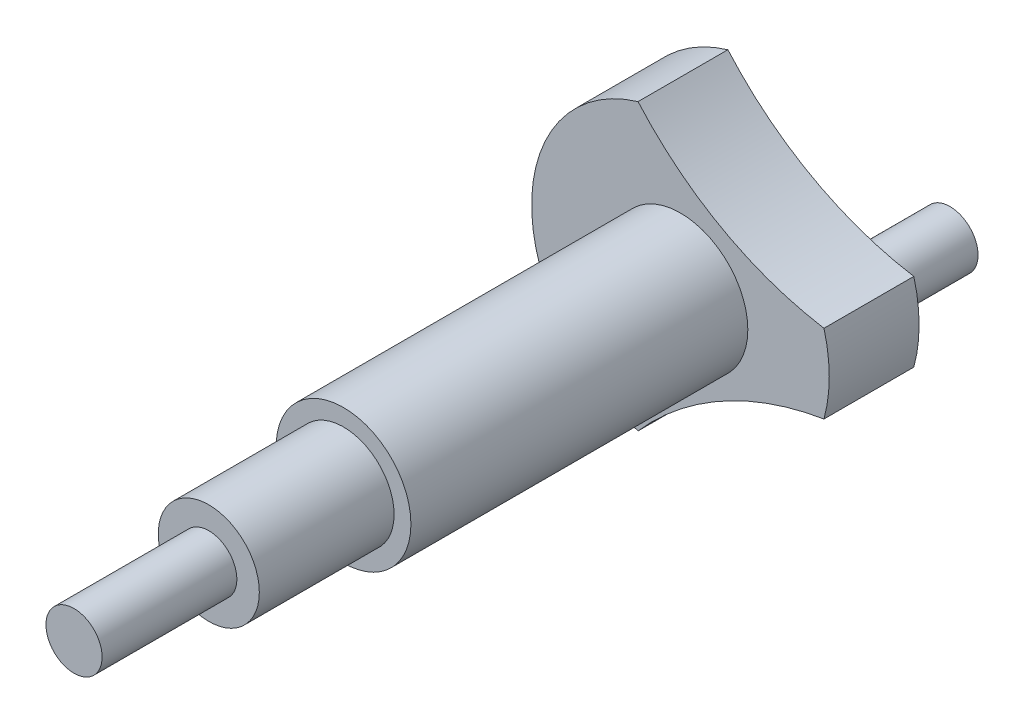
ISO-10303-21;
HEADER;
FILE_DESCRIPTION(('STEP AP214'),'2;1');
FILE_NAME('part.step','',(''),(''),'','','');
FILE_SCHEMA(('AUTOMOTIVE_DESIGN { 1 0 10303 214 1 1 1 1 }'));
ENDSEC;
DATA;
#1=APPLICATION_CONTEXT('core data for automotive mechanical design processes');
#2=APPLICATION_PROTOCOL_DEFINITION('international standard','automotive_design',2000,#1);
#3=PRODUCT_CONTEXT('',#1,'mechanical');
#4=PRODUCT('Part','Part','',(#3));
#5=PRODUCT_RELATED_PRODUCT_CATEGORY('part','',(#4));
#6=PRODUCT_DEFINITION_FORMATION('','',#4);
#7=PRODUCT_DEFINITION_CONTEXT('part definition',#1,'design');
#8=PRODUCT_DEFINITION('design','',#6,#7);
#9=PRODUCT_DEFINITION_SHAPE('','',#8);
#10=(LENGTH_UNIT() NAMED_UNIT(*) SI_UNIT(.MILLI.,.METRE.));
#11=(NAMED_UNIT(*) PLANE_ANGLE_UNIT() SI_UNIT($,.RADIAN.));
#12=(NAMED_UNIT(*) SI_UNIT($,.STERADIAN.) SOLID_ANGLE_UNIT());
#13=UNCERTAINTY_MEASURE_WITH_UNIT(LENGTH_MEASURE(1.E-05),#10,'distance_accuracy_value','');
#14=(GEOMETRIC_REPRESENTATION_CONTEXT(3) GLOBAL_UNCERTAINTY_ASSIGNED_CONTEXT((#13)) GLOBAL_UNIT_ASSIGNED_CONTEXT((#10,
#11,#12)) REPRESENTATION_CONTEXT('',''));
#15=CARTESIAN_POINT('',(0.,0.,0.));
#16=DIRECTION('',(0.,0.,1.));
#17=DIRECTION('',(1.,0.,0.));
#18=AXIS2_PLACEMENT_3D('',#15,#16,#17);
#19=CARTESIAN_POINT('',(0.,0.,30.));
#20=DIRECTION('',(0.,0.,-1.));
#21=DIRECTION('',(-1.,0.,0.));
#22=AXIS2_PLACEMENT_3D('',#19,#20,#21);
#23=CYLINDRICAL_SURFACE('',#22,6.);
#24=CARTESIAN_POINT('',(0.,0.,30.));
#25=DIRECTION('',(0.,0.,1.));
#26=DIRECTION('',(1.,0.,0.));
#27=AXIS2_PLACEMENT_3D('',#24,#25,#26);
#28=CIRCLE('',#27,6.);
#29=CARTESIAN_POINT('',(6.,0.,30.));
#30=VERTEX_POINT('',#29);
#31=EDGE_CURVE('E123',#30,#30,#28,.T.);
#32=ORIENTED_EDGE('',*,*,#31,.F.);
#33=EDGE_LOOP('',(#32));
#34=FACE_BOUND('',#33,.T.);
#35=CARTESIAN_POINT('',(0.,0.,0.));
#36=DIRECTION('',(0.,0.,1.));
#37=DIRECTION('',(1.,0.,0.));
#38=AXIS2_PLACEMENT_3D('',#35,#36,#37);
#39=CIRCLE('',#38,6.);
#40=CARTESIAN_POINT('',(6.,0.,0.));
#41=VERTEX_POINT('',#40);
#42=EDGE_CURVE('E45',#41,#41,#39,.T.);
#43=ORIENTED_EDGE('',*,*,#42,.T.);
#44=EDGE_LOOP('',(#43));
#45=FACE_BOUND('',#44,.T.);
#46=ADVANCED_FACE('F39',(#34,#45),#23,.T.);
#47=CARTESIAN_POINT('',(0.,0.,30.));
#48=DIRECTION('',(0.,0.,1.));
#49=DIRECTION('',(1.,0.,0.));
#50=AXIS2_PLACEMENT_3D('',#47,#48,#49);
#51=PLANE('',#50);
#52=CARTESIAN_POINT('',(0.,0.,30.));
#53=DIRECTION('',(0.,0.,1.));
#54=DIRECTION('',(1.,0.,0.));
#55=AXIS2_PLACEMENT_3D('',#52,#53,#54);
#56=CIRCLE('',#55,4.5);
#57=CARTESIAN_POINT('',(4.5,0.,30.));
#58=VERTEX_POINT('',#57);
#59=EDGE_CURVE('E48',#58,#58,#56,.T.);
#60=ORIENTED_EDGE('',*,*,#59,.F.);
#61=EDGE_LOOP('',(#60));
#62=FACE_BOUND('',#61,.T.);
#63=ORIENTED_EDGE('',*,*,#31,.T.);
#64=EDGE_LOOP('',(#63));
#65=FACE_BOUND('',#64,.T.);
#66=ADVANCED_FACE('F129',(#62,#65),#51,.T.);
#67=CARTESIAN_POINT('',(0.,0.,42.));
#68=DIRECTION('',(0.,0.,-1.));
#69=DIRECTION('',(-1.,0.,0.));
#70=AXIS2_PLACEMENT_3D('',#67,#68,#69);
#71=CYLINDRICAL_SURFACE('',#70,4.5);
#72=CARTESIAN_POINT('',(0.,0.,42.));
#73=DIRECTION('',(0.,0.,1.));
#74=DIRECTION('',(1.,0.,0.));
#75=AXIS2_PLACEMENT_3D('',#72,#73,#74);
#76=CIRCLE('',#75,4.5);
#77=CARTESIAN_POINT('',(4.5,0.,42.));
#78=VERTEX_POINT('',#77);
#79=EDGE_CURVE('E116',#78,#78,#76,.T.);
#80=ORIENTED_EDGE('',*,*,#79,.F.);
#81=EDGE_LOOP('',(#80));
#82=FACE_BOUND('',#81,.T.);
#83=ORIENTED_EDGE('',*,*,#59,.T.);
#84=EDGE_LOOP('',(#83));
#85=FACE_BOUND('',#84,.T.);
#86=ADVANCED_FACE('F168',(#82,#85),#71,.T.);
#87=CARTESIAN_POINT('',(0.,0.,42.));
#88=DIRECTION('',(0.,0.,1.));
#89=DIRECTION('',(1.,0.,0.));
#90=AXIS2_PLACEMENT_3D('',#87,#88,#89);
#91=PLANE('',#90);
#92=CARTESIAN_POINT('',(0.,0.,42.));
#93=DIRECTION('',(0.,0.,1.));
#94=DIRECTION('',(1.,0.,0.));
#95=AXIS2_PLACEMENT_3D('',#92,#93,#94);
#96=CIRCLE('',#95,2.5);
#97=CARTESIAN_POINT('',(2.5,0.,42.));
#98=VERTEX_POINT('',#97);
#99=EDGE_CURVE('E11',#98,#98,#96,.T.);
#100=ORIENTED_EDGE('',*,*,#99,.F.);
#101=EDGE_LOOP('',(#100));
#102=FACE_BOUND('',#101,.T.);
#103=ORIENTED_EDGE('',*,*,#79,.T.);
#104=EDGE_LOOP('',(#103));
#105=FACE_BOUND('',#104,.T.);
#106=ADVANCED_FACE('F167',(#102,#105),#91,.T.);
#107=CARTESIAN_POINT('',(0.,0.,54.));
#108=DIRECTION('',(0.,0.,-1.));
#109=DIRECTION('',(-1.,0.,0.));
#110=AXIS2_PLACEMENT_3D('',#107,#108,#109);
#111=CYLINDRICAL_SURFACE('',#110,2.5);
#112=CARTESIAN_POINT('',(0.,0.,54.));
#113=DIRECTION('',(0.,0.,1.));
#114=DIRECTION('',(1.,0.,0.));
#115=AXIS2_PLACEMENT_3D('',#112,#113,#114);
#116=CIRCLE('',#115,2.5);
#117=CARTESIAN_POINT('',(2.5,0.,54.));
#118=VERTEX_POINT('',#117);
#119=EDGE_CURVE('E117',#118,#118,#116,.T.);
#120=ORIENTED_EDGE('',*,*,#119,.F.);
#121=EDGE_LOOP('',(#120));
#122=FACE_BOUND('',#121,.T.);
#123=ORIENTED_EDGE('',*,*,#99,.T.);
#124=EDGE_LOOP('',(#123));
#125=FACE_BOUND('',#124,.T.);
#126=ADVANCED_FACE('F165',(#122,#125),#111,.T.);
#127=CARTESIAN_POINT('',(0.,0.,54.));
#128=DIRECTION('',(0.,0.,1.));
#129=DIRECTION('',(1.,0.,0.));
#130=AXIS2_PLACEMENT_3D('',#127,#128,#129);
#131=PLANE('',#130);
#132=ORIENTED_EDGE('',*,*,#119,.T.);
#133=EDGE_LOOP('',(#132));
#134=FACE_BOUND('',#133,.T.);
#135=ADVANCED_FACE('F157',(#134),#131,.T.);
#136=CARTESIAN_POINT('',(17.298973240206,31.1328293544785,-8.));
#137=DIRECTION('',(0.,0.,1.));
#138=DIRECTION('',(1.,0.,0.));
#139=AXIS2_PLACEMENT_3D('',#136,#137,#138);
#140=CYLINDRICAL_SURFACE('',#139,28.);
#141=CARTESIAN_POINT('',(17.298973240206,31.1328293544785,0.));
#142=DIRECTION('',(0.,0.,1.));
#143=DIRECTION('',(-1.,0.,0.));
#144=AXIS2_PLACEMENT_3D('',#141,#142,#143);
#145=CIRCLE('',#144,28.);
#146=CARTESIAN_POINT('',(-3.77782799653368,12.7000203003226,0.));
#147=VERTEX_POINT('',#146);
#148=CARTESIAN_POINT('',(12.7793779191321,3.5,0.));
#149=VERTEX_POINT('',#148);
#150=EDGE_CURVE('E107',#147,#149,#145,.T.);
#151=ORIENTED_EDGE('',*,*,#150,.T.);
#152=DIRECTION('',(0.,0.,1.));
#153=VECTOR('',#152,1.);
#154=CARTESIAN_POINT('',(12.7793779191321,3.5,-8.));
#155=LINE('',#154,#153);
#156=CARTESIAN_POINT('',(12.7793779191321,3.5,-8.));
#157=VERTEX_POINT('',#156);
#158=EDGE_CURVE('E97',#157,#149,#155,.T.);
#159=ORIENTED_EDGE('',*,*,#158,.F.);
#160=CARTESIAN_POINT('',(17.298973240206,31.1328293544785,-8.));
#161=DIRECTION('',(0.,0.,1.));
#162=DIRECTION('',(-1.,0.,0.));
#163=AXIS2_PLACEMENT_3D('',#160,#161,#162);
#164=CIRCLE('',#163,28.);
#165=CARTESIAN_POINT('',(-3.77782799653368,12.7000203003226,-8.));
#166=VERTEX_POINT('',#165);
#167=EDGE_CURVE('E91',#166,#157,#164,.T.);
#168=ORIENTED_EDGE('',*,*,#167,.F.);
#169=DIRECTION('',(0.,0.,1.));
#170=VECTOR('',#169,1.);
#171=CARTESIAN_POINT('',(-3.77782799653368,12.7000203003226,-8.));
#172=LINE('',#171,#170);
#173=EDGE_CURVE('E102',#166,#147,#172,.T.);
#174=ORIENTED_EDGE('',*,*,#173,.T.);
#175=EDGE_LOOP('',(#151,#159,#168,#174));
#176=FACE_BOUND('',#175,.T.);
#177=ADVANCED_FACE('F141',(#176),#140,.F.);
#178=CARTESIAN_POINT('',(0.,0.,-8.));
#179=DIRECTION('',(0.,0.,1.));
#180=DIRECTION('',(1.,0.,0.));
#181=AXIS2_PLACEMENT_3D('',#178,#179,#180);
#182=CYLINDRICAL_SURFACE('',#181,13.25);
#183=CARTESIAN_POINT('',(0.,0.,0.));
#184=DIRECTION('',(0.,0.,-1.));
#185=DIRECTION('',(-1.,0.,0.));
#186=AXIS2_PLACEMENT_3D('',#183,#184,#185);
#187=CIRCLE('',#186,13.25);
#188=CARTESIAN_POINT('',(12.7793779191321,-3.49999999999999,0.));
#189=VERTEX_POINT('',#188);
#190=EDGE_CURVE('E98',#149,#189,#187,.T.);
#191=ORIENTED_EDGE('',*,*,#190,.T.);
#192=DIRECTION('',(0.,0.,1.));
#193=VECTOR('',#192,1.);
#194=CARTESIAN_POINT('',(12.7793779191321,-3.49999999999999,-8.));
#195=LINE('',#194,#193);
#196=CARTESIAN_POINT('',(12.7793779191321,-3.49999999999999,-8.));
#197=VERTEX_POINT('',#196);
#198=EDGE_CURVE('E96',#197,#189,#195,.T.);
#199=ORIENTED_EDGE('',*,*,#198,.F.);
#200=CARTESIAN_POINT('',(0.,0.,-8.));
#201=DIRECTION('',(0.,0.,-1.));
#202=DIRECTION('',(-1.,0.,0.));
#203=AXIS2_PLACEMENT_3D('',#200,#201,#202);
#204=CIRCLE('',#203,13.25);
#205=EDGE_CURVE('E86',#157,#197,#204,.T.);
#206=ORIENTED_EDGE('',*,*,#205,.F.);
#207=ORIENTED_EDGE('',*,*,#158,.T.);
#208=EDGE_LOOP('',(#191,#199,#206,#207));
#209=FACE_BOUND('',#208,.T.);
#210=ADVANCED_FACE('F100',(#209),#182,.T.);
#211=CARTESIAN_POINT('',(17.298973240206,-31.1328293544785,-8.));
#212=DIRECTION('',(0.,0.,1.));
#213=DIRECTION('',(1.,0.,0.));
#214=AXIS2_PLACEMENT_3D('',#211,#212,#213);
#215=CYLINDRICAL_SURFACE('',#214,28.);
#216=CARTESIAN_POINT('',(17.298973240206,-31.1328293544785,0.));
#217=DIRECTION('',(0.,0.,1.));
#218=DIRECTION('',(1.,0.,0.));
#219=AXIS2_PLACEMENT_3D('',#216,#217,#218);
#220=CIRCLE('',#219,28.);
#221=CARTESIAN_POINT('',(-3.77782799653368,-12.7000203003226,0.));
#222=VERTEX_POINT('',#221);
#223=EDGE_CURVE('E74',#189,#222,#220,.T.);
#224=ORIENTED_EDGE('',*,*,#223,.T.);
#225=DIRECTION('',(0.,0.,1.));
#226=VECTOR('',#225,1.);
#227=CARTESIAN_POINT('',(-3.77782799653368,-12.7000203003226,-8.));
#228=LINE('',#227,#226);
#229=CARTESIAN_POINT('',(-3.77782799653368,-12.7000203003226,-8.));
#230=VERTEX_POINT('',#229);
#231=EDGE_CURVE('E99',#230,#222,#228,.T.);
#232=ORIENTED_EDGE('',*,*,#231,.F.);
#233=CARTESIAN_POINT('',(17.298973240206,-31.1328293544785,-8.));
#234=DIRECTION('',(0.,0.,1.));
#235=DIRECTION('',(1.,0.,0.));
#236=AXIS2_PLACEMENT_3D('',#233,#234,#235);
#237=CIRCLE('',#236,28.);
#238=EDGE_CURVE('E93',#197,#230,#237,.T.);
#239=ORIENTED_EDGE('',*,*,#238,.F.);
#240=ORIENTED_EDGE('',*,*,#198,.T.);
#241=EDGE_LOOP('',(#224,#232,#239,#240));
#242=FACE_BOUND('',#241,.T.);
#243=ADVANCED_FACE('F105',(#242),#215,.F.);
#244=CARTESIAN_POINT('',(0.,0.,-8.));
#245=DIRECTION('',(0.,0.,1.));
#246=DIRECTION('',(1.,0.,0.));
#247=AXIS2_PLACEMENT_3D('',#244,#245,#246);
#248=CYLINDRICAL_SURFACE('',#247,13.25);
#249=CARTESIAN_POINT('',(0.,0.,0.));
#250=DIRECTION('',(0.,0.,-1.));
#251=DIRECTION('',(-1.,0.,0.));
#252=AXIS2_PLACEMENT_3D('',#249,#250,#251);
#253=CIRCLE('',#252,13.25);
#254=EDGE_CURVE('E76',#222,#147,#253,.T.);
#255=ORIENTED_EDGE('',*,*,#254,.T.);
#256=ORIENTED_EDGE('',*,*,#173,.F.);
#257=CARTESIAN_POINT('',(0.,0.,-8.));
#258=DIRECTION('',(0.,0.,-1.));
#259=DIRECTION('',(-1.,0.,0.));
#260=AXIS2_PLACEMENT_3D('',#257,#258,#259);
#261=CIRCLE('',#260,13.25);
#262=EDGE_CURVE('E60',#230,#166,#261,.T.);
#263=ORIENTED_EDGE('',*,*,#262,.F.);
#264=ORIENTED_EDGE('',*,*,#231,.T.);
#265=EDGE_LOOP('',(#255,#256,#263,#264));
#266=FACE_BOUND('',#265,.T.);
#267=ADVANCED_FACE('F145',(#266),#248,.T.);
#268=CARTESIAN_POINT('',(8.64948662010298,15.5664146772392,-8.));
#269=DIRECTION('',(0.,0.,-1.));
#270=DIRECTION('',(-1.,0.,0.));
#271=AXIS2_PLACEMENT_3D('',#268,#269,#270);
#272=PLANE('',#271);
#273=CARTESIAN_POINT('',(8.,0.,-8.));
#274=DIRECTION('',(0.,0.,-1.));
#275=DIRECTION('',(-1.,0.,0.));
#276=AXIS2_PLACEMENT_3D('',#273,#274,#275);
#277=CIRCLE('',#276,2.5);
#278=CARTESIAN_POINT('',(5.5,0.,-8.));
#279=VERTEX_POINT('',#278);
#280=EDGE_CURVE('E256',#279,#279,#277,.T.);
#281=ORIENTED_EDGE('',*,*,#280,.F.);
#282=EDGE_LOOP('',(#281));
#283=FACE_BOUND('',#282,.T.);
#284=ORIENTED_EDGE('',*,*,#167,.T.);
#285=ORIENTED_EDGE('',*,*,#205,.T.);
#286=ORIENTED_EDGE('',*,*,#238,.T.);
#287=ORIENTED_EDGE('',*,*,#262,.T.);
#288=EDGE_LOOP('',(#284,#285,#286,#287));
#289=FACE_BOUND('',#288,.T.);
#290=ADVANCED_FACE('F90',(#283,#289),#272,.T.);
#291=CARTESIAN_POINT('',(8.64948662010298,15.5664146772392,0.));
#292=DIRECTION('',(0.,0.,-1.));
#293=DIRECTION('',(-1.,0.,0.));
#294=AXIS2_PLACEMENT_3D('',#291,#292,#293);
#295=PLANE('',#294);
#296=ORIENTED_EDGE('',*,*,#42,.F.);
#297=EDGE_LOOP('',(#296));
#298=FACE_BOUND('',#297,.T.);
#299=ORIENTED_EDGE('',*,*,#150,.F.);
#300=ORIENTED_EDGE('',*,*,#254,.F.);
#301=ORIENTED_EDGE('',*,*,#223,.F.);
#302=ORIENTED_EDGE('',*,*,#190,.F.);
#303=EDGE_LOOP('',(#299,#300,#301,#302));
#304=FACE_BOUND('',#303,.T.);
#305=ADVANCED_FACE('F136',(#298,#304),#295,.F.);
#306=CARTESIAN_POINT('',(8.,0.,-16.));
#307=DIRECTION('',(0.,0.,1.));
#308=DIRECTION('',(1.,0.,0.));
#309=AXIS2_PLACEMENT_3D('',#306,#307,#308);
#310=CYLINDRICAL_SURFACE('',#309,2.5);
#311=CARTESIAN_POINT('',(8.,0.,-16.));
#312=DIRECTION('',(0.,0.,-1.));
#313=DIRECTION('',(-1.,0.,0.));
#314=AXIS2_PLACEMENT_3D('',#311,#312,#313);
#315=CIRCLE('',#314,2.5);
#316=CARTESIAN_POINT('',(5.5,0.,-16.));
#317=VERTEX_POINT('',#316);
#318=EDGE_CURVE('E112',#317,#317,#315,.T.);
#319=ORIENTED_EDGE('',*,*,#318,.F.);
#320=EDGE_LOOP('',(#319));
#321=FACE_BOUND('',#320,.T.);
#322=ORIENTED_EDGE('',*,*,#280,.T.);
#323=EDGE_LOOP('',(#322));
#324=FACE_BOUND('',#323,.T.);
#325=ADVANCED_FACE('F138',(#321,#324),#310,.T.);
#326=CARTESIAN_POINT('',(8.,0.,-16.));
#327=DIRECTION('',(0.,0.,-1.));
#328=DIRECTION('',(-1.,0.,0.));
#329=AXIS2_PLACEMENT_3D('',#326,#327,#328);
#330=PLANE('',#329);
#331=ORIENTED_EDGE('',*,*,#318,.T.);
#332=EDGE_LOOP('',(#331));
#333=FACE_BOUND('',#332,.T.);
#334=ADVANCED_FACE('F242',(#333),#330,.T.);
#335=CLOSED_SHELL('',(#46,#66,#86,#106,#126,#135,#177,#210,#243,#267,#290,#305,#325,#334));
#336=MANIFOLD_SOLID_BREP('B2',#335);
#337=ADVANCED_BREP_SHAPE_REPRESENTATION('',(#18,#336),#14);
#338=SHAPE_DEFINITION_REPRESENTATION(#9,#337);
ENDSEC;
END-ISO-10303-21;
